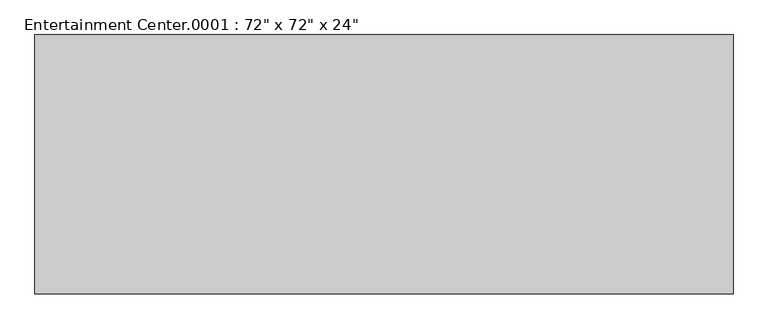
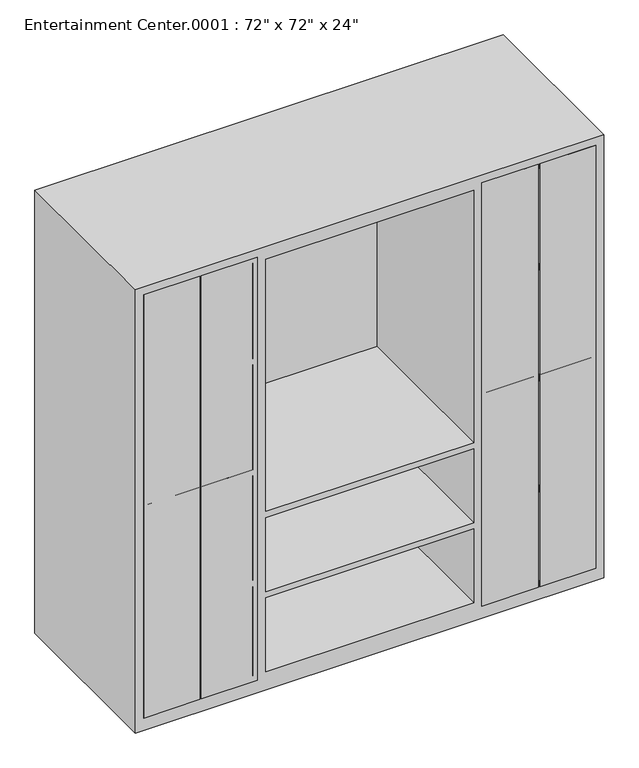
"""IFC4 building model written with IfcOpenShell, lengths in millimetres: furniture geometry."""

from ifc_helpers import new_model, si_unit, point, frame, frame_2d, origin, place, context, project, spatial, polyline, circle_curve, trimmed, segment, composite_curve, outline, extrude, faceted_brep, source, transform, mapped, element, save


def furniture_88072bd9(model_context):
    return source(origin(), model_context, "Body", "SolidModel", [
        extrude(outline(polyline([(-882.65, -711.2), (-663.575, -711.2), (-663.575, -781.05), (-882.65, -781.05), (-882.65, -711.2)])), frame((0.0, 0.0, 50.8), z_axis=(0.0, 0.0, 1.0), x_axis=(1.0, 0.0, 0.0)), (0.0, 0.0, 1.0), 1746.25),
        extrude(outline(polyline([(-657.225, -711.2), (-438.15, -711.2), (-438.15, -781.05), (-657.225, -781.05), (-657.225, -711.2)])), frame((0.0, 0.0, 50.8), z_axis=(0.0, 0.0, 1.0), x_axis=(1.0, 0.0, 0.0)), (0.0, 0.0, 1.0), 1746.25),
        extrude(outline(polyline([(663.575, -711.2), (882.65, -711.2), (882.65, -781.05), (663.575, -781.05), (663.575, -711.2)])), frame((0.0, 0.0, 50.8), z_axis=(0.0, 0.0, 1.0), x_axis=(1.0, 0.0, 0.0)), (0.0, 0.0, 1.0), 1746.25),
        extrude(outline(polyline([(438.15, -711.2), (657.225, -711.2), (657.225, -781.05), (438.15, -781.05), (438.15, -711.2)])), frame((0.0, 0.0, 50.8), z_axis=(0.0, 0.0, 1.0), x_axis=(1.0, 0.0, 0.0)), (0.0, 0.0, 1.0), 1746.25),
        extrude(outline(composite_curve([segment(polyline([(1003.3, -632.9986452), (1003.3, -657.225), (825.5, -657.225), (825.5, -632.9986452)]), True, "CONTINUOUS"), segment(trimmed(circle_curve(frame_2d((850.9, -632.9986452)), 25.4), [point((825.5, -632.9986452))], [point((850.9, -607.5986452))], False, "CARTESIAN"), True, "CONTINUOUS"), segment(polyline([(850.9, -607.5986452), (977.9, -607.5986452)]), True, "CONTINUOUS"), segment(trimmed(circle_curve(frame_2d((977.9, -632.9986452)), 25.4), [point((977.9, -607.5986452))], [point((1003.3, -632.9986452))], False, "CARTESIAN"), True, "CONTINUOUS")], self_intersect=False)), frame((0.0, -714.375, 0.0), z_axis=(0.0, 1.0, 0.0), x_axis=(0.0, 0.0, 1.0)), (0.0, 0.0, 1.0), 3.175),
        extrude(outline(composite_curve([segment(trimmed(circle_curve(frame_2d((977.9, -688.18125)), 25.4), [point((1003.3, -688.18125))], [point((977.9, -713.58125))], False, "CARTESIAN"), True, "CONTINUOUS"), segment(polyline([(977.9, -713.58125), (850.9, -713.58125)]), True, "CONTINUOUS"), segment(trimmed(circle_curve(frame_2d((850.9, -688.18125)), 25.4), [point((850.9, -713.58125))], [point((825.5, -688.18125))], False, "CARTESIAN"), True, "CONTINUOUS"), segment(polyline([(825.5, -688.18125), (825.5, -663.575), (1003.3, -663.575), (1003.3, -688.18125)]), True, "CONTINUOUS")], self_intersect=False)), frame((0.0, -714.375, 0.0), z_axis=(0.0, 1.0, 0.0), x_axis=(0.0, 0.0, 1.0)), (0.0, 0.0, 1.0), 3.175),
        extrude(outline(composite_curve([segment(trimmed(circle_curve(frame_2d((977.9, 632.9986452)), 25.4), [point((1003.3, 632.9986452))], [point((977.9, 607.5986452))], False, "CARTESIAN"), True, "CONTINUOUS"), segment(polyline([(977.9, 607.5986452), (850.9, 607.5986452)]), True, "CONTINUOUS"), segment(trimmed(circle_curve(frame_2d((850.9, 632.9986452)), 25.4), [point((850.9, 607.5986452))], [point((825.5, 632.9986452))], False, "CARTESIAN"), True, "CONTINUOUS"), segment(polyline([(825.5, 632.9986452), (825.5, 657.225), (1003.3, 657.225), (1003.3, 632.9986452)]), True, "CONTINUOUS")], self_intersect=False)), frame((0.0, -714.375, 0.0), z_axis=(0.0, 1.0, 0.0), x_axis=(0.0, 0.0, 1.0)), (0.0, 0.0, 1.0), 3.175),
        extrude(outline(composite_curve([segment(polyline([(1003.3, 688.18125), (1003.3, 663.575), (825.5, 663.575), (825.5, 688.18125)]), True, "CONTINUOUS"), segment(trimmed(circle_curve(frame_2d((850.9, 688.18125)), 25.4), [point((825.5, 688.18125))], [point((850.9, 713.58125))], False, "CARTESIAN"), True, "CONTINUOUS"), segment(polyline([(850.9, 713.58125), (977.9, 713.58125)]), True, "CONTINUOUS"), segment(trimmed(circle_curve(frame_2d((977.9, 688.18125)), 25.4), [point((977.9, 713.58125))], [point((1003.3, 688.18125))], False, "CARTESIAN"), True, "CONTINUOUS")], self_intersect=False)), frame((0.0, -714.375, 0.0), z_axis=(0.0, 1.0, 0.0), x_axis=(0.0, 0.0, 1.0)), (0.0, 0.0, 1.0), 3.175),
        faceted_brep([(914.4, -781.05, 0.0), (914.4, -781.05, 1828.8), (-914.4, -781.05, 1828.8), (-914.4, -781.05, 0.0), (-457.2, -781.05, 1778.0), (-457.2, -781.05, 1384.3), (-863.6, -781.05, 1384.3), (-863.6, -781.05, 1778.0), (-457.2, -781.05, 76.2), (-863.6, -781.05, 76.2), (-863.6, -781.05, 444.5), (-457.2, -781.05, 444.5), (863.6, -781.05, 1384.3), (457.2, -781.05, 1384.3), (457.2, -781.05, 1778.0), (863.6, -781.05, 1778.0), (-406.4, -781.05, 736.6), (-406.4, -781.05, 1778.0), (406.4, -781.05, 1778.0), (406.4, -781.05, 736.6), (406.4, -781.05, 76.2), (-406.4, -781.05, 76.2), (-406.4, -781.05, 381.0), (406.4, -781.05, 381.0), (863.6, -781.05, 76.2), (457.2, -781.05, 76.2), (457.2, -781.05, 444.5), (863.6, -781.05, 444.5), (-863.6, -781.05, 469.9), (-863.6, -781.05, 901.7), (-457.2, -781.05, 901.7), (-457.2, -781.05, 469.9), (-457.2, -781.05, 1358.9), (-457.2, -781.05, 927.1), (-863.6, -781.05, 927.1), (-863.6, -781.05, 1358.9), (457.2, -781.05, 1358.9), (863.6, -781.05, 1358.9), (863.6, -781.05, 927.1), (457.2, -781.05, 927.1), (457.2, -781.05, 901.7), (863.6, -781.05, 901.7), (863.6, -781.05, 469.9), (457.2, -781.05, 469.9), (406.4, -781.05, 406.4), (-406.4, -781.05, 406.4), (-406.4, -781.05, 711.2), (406.4, -781.05, 711.2), (914.4, -101.6, 0.0), (-914.4, -101.6, 0.0), (-914.4, -101.6, 1828.8), (914.4, -101.6, 1828.8), (-457.2, -127.0, 1778.0), (-457.2, -127.0, 1384.3), (-863.6, -127.0, 1384.3), (-863.6, -127.0, 1778.0), (-457.2, -127.0, 76.2), (-863.6, -127.0, 76.2), (-863.6, -127.0, 444.5), (-457.2, -127.0, 444.5), (863.6, -127.0, 1384.3), (457.2, -127.0, 1384.3), (457.2, -127.0, 1778.0), (863.6, -127.0, 1778.0), (-406.4, -127.0, 736.6), (-406.4, -127.0, 1778.0), (406.4, -127.0, 1778.0), (406.4, -127.0, 736.6), (406.4, -127.0, 76.2), (-406.4, -127.0, 76.2), (-406.4, -127.0, 381.0), (406.4, -127.0, 381.0), (863.6, -127.0, 76.2), (457.2, -127.0, 76.2), (457.2, -127.0, 444.5), (863.6, -127.0, 444.5), (-863.6, -127.0, 469.9), (-863.6, -127.0, 901.7), (-457.2, -127.0, 901.7), (-457.2, -127.0, 469.9), (-457.2, -127.0, 1358.9), (-457.2, -127.0, 927.1), (-863.6, -127.0, 927.1), (-863.6, -127.0, 1358.9), (457.2, -127.0, 1358.9), (863.6, -127.0, 1358.9), (863.6, -127.0, 927.1), (457.2, -127.0, 927.1), (457.2, -127.0, 901.7), (863.6, -127.0, 901.7), (863.6, -127.0, 469.9), (457.2, -127.0, 469.9), (406.4, -127.0, 406.4), (-406.4, -127.0, 406.4), (-406.4, -127.0, 711.2), (406.4, -127.0, 711.2)], [[[0, 1, 2, 3], [4, 5, 6, 7], [8, 9, 10, 11], [12, 13, 14, 15], [16, 17, 18, 19], [20, 21, 22, 23], [24, 25, 26, 27], [28, 29, 30, 31], [32, 33, 34, 35], [36, 37, 38, 39], [40, 41, 42, 43], [44, 45, 46, 47]], [[48, 49, 50, 51]], [[1, 0, 48, 51]], [[2, 1, 51, 50]], [[3, 2, 50, 49]], [[0, 3, 49, 48]], [[5, 4, 52, 53]], [[6, 5, 53, 54]], [[7, 6, 54, 55]], [[4, 7, 55, 52]], [[9, 8, 56, 57]], [[10, 9, 57, 58]], [[11, 10, 58, 59]], [[8, 11, 59, 56]], [[13, 12, 60, 61]], [[14, 13, 61, 62]], [[15, 14, 62, 63]], [[12, 15, 63, 60]], [[17, 16, 64, 65]], [[18, 17, 65, 66]], [[19, 18, 66, 67]], [[16, 19, 67, 64]], [[21, 20, 68, 69]], [[22, 21, 69, 70]], [[23, 22, 70, 71]], [[20, 23, 71, 68]], [[25, 24, 72, 73]], [[26, 25, 73, 74]], [[27, 26, 74, 75]], [[24, 27, 75, 72]], [[29, 28, 76, 77]], [[30, 29, 77, 78]], [[31, 30, 78, 79]], [[28, 31, 79, 76]], [[33, 32, 80, 81]], [[34, 33, 81, 82]], [[35, 34, 82, 83]], [[32, 35, 83, 80]], [[37, 36, 84, 85]], [[38, 37, 85, 86]], [[39, 38, 86, 87]], [[36, 39, 87, 84]], [[41, 40, 88, 89]], [[42, 41, 89, 90]], [[43, 42, 90, 91]], [[40, 43, 91, 88]], [[45, 44, 92, 93]], [[46, 45, 93, 94]], [[47, 46, 94, 95]], [[44, 47, 95, 92]], [[53, 52, 55, 54]], [[57, 56, 59, 58]], [[61, 60, 63, 62]], [[65, 64, 67, 66]], [[69, 68, 71, 70]], [[73, 72, 75, 74]], [[77, 76, 79, 78]], [[81, 80, 83, 82]], [[85, 84, 87, 86]], [[89, 88, 91, 90]], [[93, 92, 95, 94]]]),
    ])


if __name__ == "__main__":
    model = new_model("IFC4")
    model_context = context("Model", 3, world=origin())
    ifc_project = project(units=[si_unit("LENGTHUNIT", "METRE", prefix="MILLI")], contexts=[model_context])
    site = spatial("IfcSite", under=ifc_project)
    building = spatial("IfcBuilding", under=site)
    placement = place(None, origin())
    furniture_shape = furniture_88072bd9(model_context)
    element("IfcFurniture", 1, ObjectType="Entertainment Center.0001 : 72\" x 72\" x 24\"", at=placement, inside=building, context=model_context, shape_type="MappedRepresentation", body=[
        mapped(furniture_shape, transform((0.0, 0.0, 0.0), x_axis=(1.0, 0.0, 0.0), y_axis=(0.0, 1.0, 0.0), z_axis=(0.0, 0.0, 1.0))),
    ])
    save(model, "model.ifc")

# Revit data of these elements
# Type "Entertainment Center.0001 : 72\" x 72\" x 24\""
#   Assembly Code = "E2020200"
#   Center Width = 2.666667 ft
#   Depth = 2 ft
#   Height = 6 ft
#   Width = 6 ft
#   Material = none
#   Default Elevation = 0
# Element 1 (IfcFurniture, "Entertainment Center.0001 : 72\" x 72\" x 24\"")
#   Materials on its faces: "Steel, Chrome Plated", "Glass - Clear, Grey"
# Materials
#   "Steel, Chrome Plated": class "Metal", colour RGB 17 17 17, transparency 0, Description = "Chromiuim plated steel", Cost = 0
#   "Glass - Clear, Grey": class "Glass", colour RGB 252 255 255, transparency 0.64
